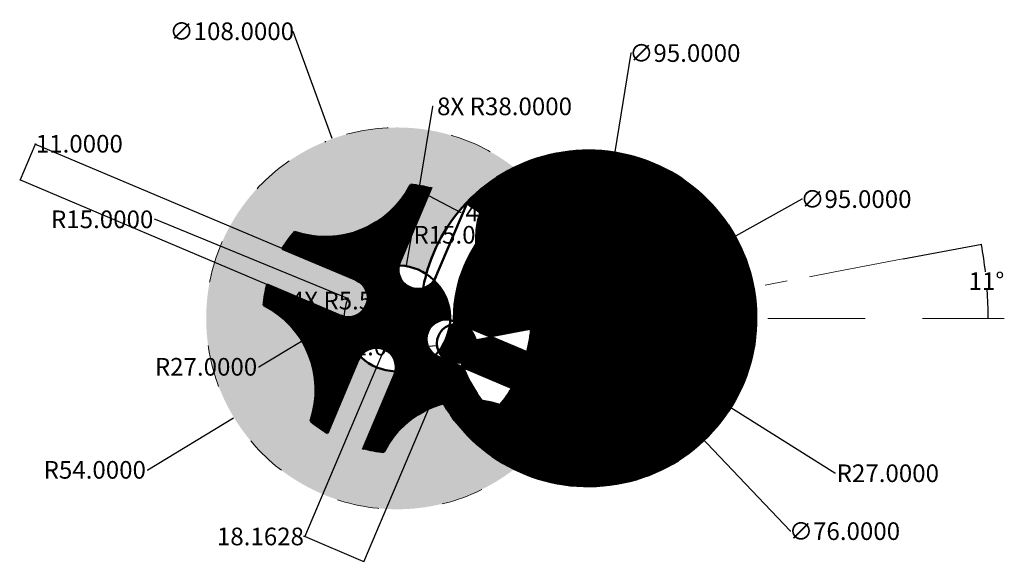
# Model space of a CAD drawing. Units: inches. Extents: x 60331 to 60609, y 22624 to 22778.
import ezdxf

# ---------------------------------------------------------------- set-up
doc = ezdxf.new("R2010")
doc.units = ezdxf.units.IN
doc.header["$MEASUREMENT"] = 0
doc.linetypes.add('ACAD_ISO03W100', pattern=[30, 12, -18])
doc.linetypes.add('CENTER', pattern=[50.8, 31.75, -6.35, 6.35, -6.35])
for name, color, linetype, lineweight in [('M-CNTR', 4, 'CENTER', 18), ('M-CONS', 8, 'ACAD_ISO03W100', 13), ('M-DIMS', 2, 'Continuous', 25), ('M-HATC', 252, 'Continuous', 18), ('M-OUTL', 7, 'Continuous', 50)]:
    doc.layers.add(name, color=color, linetype=linetype, lineweight=lineweight)
doc.styles.get("Standard").update_dxf_attribs({"font": 'arial.ttf'})
doc.dimstyles.get("Standard").update_dxf_attribs({"dimtxt": 5, "dimasz": 0.18, "dimexe": 0.18, "dimexo": 0.0625, "dimgap": 0.09, "dimtad": 0, "dimtih": 1, "dimtoh": 1, "dimdec": 4, "dimzin": 0, "dimdsep": 46, "dimtxsty": 'Standard', "dimcen": 0.09, "dimadec": 0, "dimazin": 0, "dimtfac": 1, "dimtdec": 4, "dimtofl": 0, "dimtmove": 0, "dimatfit": 3, "dimfxl": 1, "dimtolj": 1, "dimtzin": 0, "dimarcsym": 0})

# ---------------------------------------------------------------- blocks, each defined once
blk = doc.blocks.new('*D1')
at = {"layer": 'Defpoints', "color": 0, "transparency": 16777216}
for p in [(60532.97, 22716.4), (60450.04, 22670.06)]:
    blk.add_point(p, dxfattribs=at)
at = {"layer": 'M-DIMS', "color": 0, "lineweight": -2, "transparency": 16777216}
for p, q in [((60551.88, 22726.97), (60533.12, 22716.49)), ((60552.06, 22726.97), (60551.88, 22726.97)), ((60491.41, 22693.23), (60491.59, 22693.23)), ((60491.5, 22693.14), (60491.5, 22693.32))]:
    blk.add_line(p, q, dxfattribs=at)
at = {"layer": 'M-DIMS', "color": 0, "transparency": 16777216}
blk.add_solid([(60533.11, 22716.52), (60533.14, 22716.46), (60532.97, 22716.4)], dxfattribs=at)
at = {"layer": 'M-DIMS', "color": 0, "transparency": 16777216, "insert": (60567.18, 22726.97), "char_height": 5, "attachment_point": 5}
blk.add_mtext('\\A1;∅95.0000', dxfattribs=at)
blk = doc.blocks.new('*D2')
at = {"layer": 'Defpoints', "color": 0, "transparency": 16777216}
for p in [(60580.44, 22710.03), (60561.22, 22706.39), (60604.35, 22700.25), (60586.01, 22693.22), (60609.08, 22693.22)]:
    blk.add_point(p, dxfattribs=at)
at = {"layer": 'M-DIMS', "color": 0, "lineweight": -2, "transparency": 16777216}
blk.add_line((60580.5, 22710.04), (60602.78, 22714.25), dxfattribs=at)
for start, end in [(6.6776, 10.6133), (0.0912, 4.0298)]:
    blk.add_arc((60491.54, 22693.22), 113.04, start, end, dxfattribs=at)
at = {"layer": 'M-DIMS', "color": 0, "transparency": 16777216}
for points in [[(60602.61, 22714.03), (60602.67, 22714.04), (60602.61, 22714.22)], [(60604.6, 22693.4), (60604.54, 22693.4), (60604.57, 22693.22)]]:
    blk.add_solid(points, dxfattribs=at)
at = {"layer": 'M-DIMS', "color": 0, "transparency": 16777216, "insert": (60604.08, 22703.76), "char_height": 5, "attachment_point": 5}
blk.add_mtext('\\A1;11°', dxfattribs=at)
blk = doc.blocks.new('*D3')
at = {"layer": 'Defpoints', "color": 0, "transparency": 16777216}
for p in [(60491.5, 22693.23), (60514.36, 22678.87)]:
    blk.add_point(p, dxfattribs=at)
at = {"layer": 'M-DIMS', "color": 0, "lineweight": -2, "transparency": 16777216}
for p, q in [((60491.41, 22693.23), (60491.59, 22693.23)), ((60491.5, 22693.14), (60491.5, 22693.32)), ((60561.22, 22649.42), (60514.52, 22678.77)), ((60561.4, 22649.42), (60561.22, 22649.42))]:
    blk.add_line(p, q, dxfattribs=at)
at = {"layer": 'M-DIMS', "color": 0, "transparency": 16777216}
blk.add_solid([(60514.53, 22678.8), (60514.5, 22678.74), (60514.36, 22678.87)], dxfattribs=at)
at = {"layer": 'M-DIMS', "color": 0, "transparency": 16777216, "insert": (60576.19, 22649.42), "char_height": 5, "attachment_point": 5}
blk.add_mtext('\\A1;R27.0000', dxfattribs=at)
blk = doc.blocks.new('*D4')
at = {"layer": 'Defpoints', "color": 0, "transparency": 16777216}
for p in [(60465.34, 22720.79), (60517.66, 22665.67)]:
    blk.add_point(p, dxfattribs=at)
at = {"layer": 'M-DIMS', "color": 0, "lineweight": -2, "transparency": 16777216}
for p, q in [((60491.41, 22693.23), (60491.59, 22693.23)), ((60491.5, 22693.14), (60491.5, 22693.32)), ((60548.63, 22633.04), (60517.79, 22665.54)), ((60548.81, 22633.04), (60548.63, 22633.04))]:
    blk.add_line(p, q, dxfattribs=at)
at = {"layer": 'M-DIMS', "color": 0, "transparency": 16777216}
blk.add_solid([(60517.81, 22665.56), (60517.76, 22665.52), (60517.66, 22665.67)], dxfattribs=at)
at = {"layer": 'M-DIMS', "color": 0, "transparency": 16777216, "insert": (60563.94, 22633.04), "char_height": 5, "attachment_point": 5}
blk.add_mtext('\\A1;∅76.0000', dxfattribs=at)
blk = doc.blocks.new('*D5')
at = {"layer": 'Defpoints', "color": 0, "transparency": 16777216}
for p in [(60437.44, 22693.23), (60454.17, 22686.16), (60411.31, 22631.47)]:
    blk.add_point(p, dxfattribs=at)
at = {"layer": 'M-DIMS', "color": 0, "lineweight": -2, "transparency": 16777216}
for p, q in [((60437.41, 22693.17), (60411.24, 22631.3)), ((60454.14, 22686.1), (60427.97, 22624.23)), ((60411.15, 22631.54), (60410.97, 22631.54)), ((60411.31, 22631.47), (60411.15, 22631.54)), ((60427.87, 22624.46), (60411.48, 22631.4))]:
    blk.add_line(p, q, dxfattribs=at)
at = {"layer": 'M-DIMS', "color": 0, "transparency": 16777216}
for points in [[(60411.49, 22631.43), (60411.47, 22631.37), (60411.31, 22631.47)], [(60427.89, 22624.49), (60427.86, 22624.43), (60428.04, 22624.39)]]:
    blk.add_solid(points, dxfattribs=at)
at = {"layer": 'M-DIMS', "color": 0, "transparency": 16777216, "insert": (60398.79, 22631.54), "char_height": 5, "attachment_point": 5}
blk.add_mtext('\\A1;18.1628', dxfattribs=at)
blk = doc.blocks.new('*D6')
at = {"layer": 'Defpoints', "color": 0, "transparency": 16777216}
for p in [(60423.56, 22698.92), (60437.44, 22693.23)]:
    blk.add_point(p, dxfattribs=at)
at = {"layer": 'M-DIMS', "color": 0, "lineweight": -2, "transparency": 16777216}
for p, q in [((60368.83, 22721.25), (60369.01, 22721.25)), ((60369.01, 22721.25), (60423.39, 22698.98)), ((60437.35, 22693.23), (60437.53, 22693.23)), ((60437.44, 22693.14), (60437.44, 22693.32))]:
    blk.add_line(p, q, dxfattribs=at)
blk.add_arc((60437.44, 22693.23), 15, 157.0434, 177.9603, dxfattribs=at)
at = {"layer": 'M-DIMS', "color": 0, "transparency": 16777216}
blk.add_solid([(60423.4, 22699.01), (60423.38, 22698.96), (60423.56, 22698.92)], dxfattribs=at)
at = {"layer": 'M-DIMS', "color": 0, "transparency": 16777216, "insert": (60354.03, 22721.25), "char_height": 5, "attachment_point": 5}
blk.add_mtext('\\A1;R15.0000', dxfattribs=at)
blk = doc.blocks.new('*D7')
at = {"layer": 'Defpoints', "color": 0, "transparency": 16777216}
for p in [(60410.55, 22686.83), (60387.4, 22672.94)]:
    blk.add_point(p, dxfattribs=at)
at = {"layer": 'M-DIMS', "color": 0, "lineweight": -2, "transparency": 16777216}
for p, q in [((60398.37, 22679.53), (60410.39, 22686.74)), ((60398.19, 22679.53), (60398.37, 22679.53))]:
    blk.add_line(p, q, dxfattribs=at)
at = {"layer": 'M-DIMS', "color": 0, "transparency": 16777216}
blk.add_solid([(60410.38, 22686.76), (60410.41, 22686.71), (60410.55, 22686.83)], dxfattribs=at)
at = {"layer": 'M-DIMS', "color": 0, "transparency": 16777216, "insert": (60383.4, 22679.53), "char_height": 5, "attachment_point": 5}
blk.add_mtext('\\A1;R27.0000', dxfattribs=at)
blk = doc.blocks.new('*D8')
at = {"layer": 'Defpoints', "color": 0, "transparency": 16777216}
for p in [(60437.44, 22693.23), (60391.29, 22665.19)]:
    blk.add_point(p, dxfattribs=at)
at = {"layer": 'M-DIMS', "color": 0, "lineweight": -2, "transparency": 16777216}
for p, q in [((60437.35, 22693.23), (60437.53, 22693.23)), ((60437.44, 22693.14), (60437.44, 22693.32)), ((60366.91, 22650.38), (60391.14, 22665.1)), ((60366.73, 22650.38), (60366.91, 22650.38))]:
    blk.add_line(p, q, dxfattribs=at)
at = {"layer": 'M-DIMS', "color": 0, "transparency": 16777216}
blk.add_solid([(60391.12, 22665.12), (60391.15, 22665.07), (60391.29, 22665.19)], dxfattribs=at)
at = {"layer": 'M-DIMS', "color": 0, "transparency": 16777216, "insert": (60351.94, 22650.38), "char_height": 5, "attachment_point": 5}
blk.add_mtext('\\A1;R54.0000', dxfattribs=at)
blk = doc.blocks.new('*D9')
at = {"layer": 'Defpoints', "color": 0, "transparency": 16777216}
for p in [(60335.16, 22742.47), (60404.95, 22712.95), (60400.67, 22702.81)]:
    blk.add_point(p, dxfattribs=at)
at = {"layer": 'M-DIMS', "color": 0, "lineweight": -2, "transparency": 16777216}
for p, q in [((60330.95, 22732.5), (60335.09, 22742.3)), ((60404.9, 22712.97), (60335, 22742.54)), ((60335.16, 22742.47), (60335.23, 22742.63)), ((60335.23, 22742.63), (60335.41, 22742.63)), ((60400.61, 22702.84), (60330.71, 22732.41))]:
    blk.add_line(p, q, dxfattribs=at)
at = {"layer": 'M-DIMS', "color": 0, "transparency": 16777216}
for points in [[(60335.06, 22742.31), (60335.12, 22742.29), (60335.16, 22742.47)], [(60330.92, 22732.51), (60330.97, 22732.49), (60330.88, 22732.34)]]:
    blk.add_solid(points, dxfattribs=at)
at = {"layer": 'M-DIMS', "color": 0, "transparency": 16777216, "insert": (60347.58, 22742.63), "char_height": 5, "attachment_point": 5}
blk.add_mtext('\\A1;11.0000', dxfattribs=at)
blk = doc.blocks.new('*D10')
at = {"layer": 'Defpoints', "color": 0, "transparency": 16777216}
for p in [(60419, 22743.99), (60455.88, 22642.48)]:
    blk.add_point(p, dxfattribs=at)
at = {"layer": 'M-DIMS', "color": 0, "lineweight": -2, "transparency": 16777216}
for p, q in [((60407.76, 22774.44), (60407.94, 22774.44)), ((60407.94, 22774.44), (60418.94, 22744.16)), ((60437.35, 22693.23), (60437.53, 22693.23)), ((60437.44, 22693.14), (60437.44, 22693.32))]:
    blk.add_line(p, q, dxfattribs=at)
at = {"layer": 'M-DIMS', "color": 0, "transparency": 16777216}
blk.add_solid([(60418.97, 22744.17), (60418.91, 22744.15), (60419, 22743.99)], dxfattribs=at)
at = {"layer": 'M-DIMS', "color": 0, "transparency": 16777216, "insert": (60390.69, 22774.44), "char_height": 5, "attachment_point": 5}
blk.add_mtext('\\A1;∅108.0000', dxfattribs=at)
blk = doc.blocks.new('*D11')
at = {"layer": 'Defpoints', "color": 0, "transparency": 16777216}
for p in [(60499, 22740.14), (60484, 22646.33)]:
    blk.add_point(p, dxfattribs=at)
at = {"layer": 'M-DIMS', "color": 0, "lineweight": -2, "transparency": 16777216}
for p, q in [((60503.5, 22768.28), (60499.03, 22740.31)), ((60503.68, 22768.28), (60503.5, 22768.28)), ((60491.41, 22693.23), (60491.59, 22693.23)), ((60491.5, 22693.14), (60491.5, 22693.32))]:
    blk.add_line(p, q, dxfattribs=at)
at = {"layer": 'M-DIMS', "color": 0, "transparency": 16777216}
blk.add_solid([(60499, 22740.32), (60499.06, 22740.31), (60499, 22740.14)], dxfattribs=at)
at = {"layer": 'M-DIMS', "color": 0, "transparency": 16777216, "insert": (60518.8, 22768.28), "char_height": 5, "attachment_point": 5}
blk.add_mtext('\\A1;∅95.0000', dxfattribs=at)
blk = doc.blocks.new('*D12')
at = {"layer": 'Defpoints', "color": 0, "transparency": 16777216}
for p in [(60417.15, 22743.27), (60441.04, 22730.7)]:
    blk.add_point(p, dxfattribs=at)
at = {"layer": 'M-DIMS', "color": 0, "lineweight": -2, "transparency": 16777216}
for p, q in [((60417.06, 22743.27), (60417.24, 22743.27)), ((60417.15, 22743.18), (60417.15, 22743.36)), ((60455.38, 22723.16), (60441.2, 22730.62)), ((60455.56, 22723.16), (60455.38, 22723.16))]:
    blk.add_line(p, q, dxfattribs=at)
at = {"layer": 'M-DIMS', "color": 0, "transparency": 16777216}
blk.add_solid([(60441.22, 22730.64), (60441.19, 22730.59), (60441.04, 22730.7)], dxfattribs=at)
at = {"layer": 'M-DIMS', "color": 0, "transparency": 16777216, "insert": (60475.83, 22723.16), "char_height": 5, "attachment_point": 5}
blk.add_mtext('\\A1;4X R27.0000', dxfattribs=at)
blk = doc.blocks.new('*D13')
at = {"layer": 'Defpoints', "color": 0, "transparency": 16777216}
for p in [(60440, 22708.01), (60437.44, 22693.23)]:
    blk.add_point(p, dxfattribs=at)
at = {"layer": 'M-DIMS', "color": 0, "lineweight": -2, "transparency": 16777216}
for p, q in [((60441.54, 22716.88), (60440.03, 22708.19)), ((60441.72, 22716.88), (60441.54, 22716.88)), ((60437.35, 22693.23), (60437.53, 22693.23)), ((60437.44, 22693.14), (60437.44, 22693.32))]:
    blk.add_line(p, q, dxfattribs=at)
at = {"layer": 'M-DIMS', "color": 0, "transparency": 16777216}
blk.add_solid([(60440, 22708.19), (60440.06, 22708.18), (60440, 22708.01)], dxfattribs=at)
at = {"layer": 'M-DIMS', "color": 0, "transparency": 16777216, "insert": (60456.51, 22716.88), "char_height": 5, "attachment_point": 5}
blk.add_mtext('\\A1;R15.0000', dxfattribs=at)
blk = doc.blocks.new('*D14')
at = {"layer": 'Defpoints', "color": 0, "transparency": 16777216}
for p in [(60443.28, 22707.05), (60443.15, 22701.55)]:
    blk.add_point(p, dxfattribs=at)
at = {"layer": 'M-DIMS', "color": 0, "lineweight": -2, "transparency": 16777216}
for p, q in [((60443.19, 22707.05), (60443.37, 22707.05)), ((60443.28, 22706.96), (60443.28, 22707.14)), ((60443.07, 22698.25), (60443.14, 22701.37)), ((60442.89, 22698.25), (60443.07, 22698.25))]:
    blk.add_line(p, q, dxfattribs=at)
at = {"layer": 'M-DIMS', "color": 0, "transparency": 16777216}
blk.add_solid([(60443.11, 22701.37), (60443.17, 22701.37), (60443.15, 22701.55)], dxfattribs=at)
at = {"layer": 'M-DIMS', "color": 0, "transparency": 16777216, "insert": (60424.56, 22698.25), "char_height": 5, "attachment_point": 5}
blk.add_mtext('\\A1;4X R5.5000', dxfattribs=at)
blk = doc.blocks.new('*D15')
at = {"layer": 'Defpoints', "color": 0, "transparency": 16777216}
for p in [(60448.69, 22685.6), (60459.64, 22686.71)]:
    blk.add_point(p, dxfattribs=at)
at = {"layer": 'M-DIMS', "color": 0, "lineweight": -2, "transparency": 16777216}
for p, q in [((60445.41, 22685.27), (60448.52, 22685.58)), ((60454.08, 22686.16), (60454.26, 22686.16)), ((60454.17, 22686.07), (60454.17, 22686.25))]:
    blk.add_line(p, q, dxfattribs=at)
at = {"layer": 'M-DIMS', "color": 0, "transparency": 16777216}
blk.add_solid([(60448.51, 22685.61), (60448.52, 22685.55), (60448.69, 22685.6)], dxfattribs=at)
at = {"layer": 'M-DIMS', "color": 0, "transparency": 16777216, "insert": (60430.29, 22685.27), "char_height": 5, "attachment_point": 5}
blk.add_mtext('\\A1;∅11.0000', dxfattribs=at)
blk = doc.blocks.new('*D16')
at = {"layer": 'Defpoints', "color": 0, "transparency": 16777216}
for p in [(60443.7, 22730.71), (60437.44, 22693.23)]:
    blk.add_point(p, dxfattribs=at)
at = {"layer": 'M-DIMS', "color": 0, "lineweight": -2, "transparency": 16777216}
for p, q in [((60447.46, 22753.2), (60443.73, 22730.89)), ((60447.64, 22753.2), (60447.46, 22753.2)), ((60437.35, 22693.23), (60437.53, 22693.23)), ((60437.44, 22693.14), (60437.44, 22693.32))]:
    blk.add_line(p, q, dxfattribs=at)
at = {"layer": 'M-DIMS', "color": 0, "transparency": 16777216}
blk.add_solid([(60443.7, 22730.89), (60443.76, 22730.88), (60443.7, 22730.71)], dxfattribs=at)
at = {"layer": 'M-DIMS', "color": 0, "transparency": 16777216, "insert": (60467.81, 22753.2), "char_height": 5, "attachment_point": 5}
blk.add_mtext('\\A1;8X R38.0000', dxfattribs=at)

msp = doc.modelspace()

# ---------------------------------------------------------------- hatches: boundary and pattern name
at = {"layer": 'M-HATC'}
h = msp.add_hatch(color=256, dxfattribs=at)
h.dxf.hatch_style = 1
h.paths.add_polyline_path([(60383.4389, 22693.23138, 0.62395168), (60470.57212, 22650.59115, -0.147115616), (60450.52409, 22669.20932, 0.210663072), (60433.65907, 22655.41984, -0.038845732), (60427.85582, 22656.45959), (60436.66049, 22677.27381, 0.04612672), (60436.96747, 22678.23879, -0.186494261), (60427.00831, 22682.45164, 0.04612672), (60426.52962, 22681.5593), (60417.72495, 22660.74508, -0.038845732), (60412.93719, 22664.18545, 0.373805178), (60399.62735, 22697.01121, -0.038845732), (60400.66711, 22702.81446), (60421.48133, 22694.00979, 0.04612672), (60422.44631, 22693.70281, 0.911814278), (60425.76681, 22704.14066), (60404.95259, 22712.94533, -0.038845732), (60408.39296, 22717.73309, 0.373805178), (60441.21873, 22731.04293, -0.038845732), (60447.02197, 22730.00318), (60438.2173, 22709.18896, 0.04612672), (60437.91032, 22708.22398, -0.138521755), (60445.68454, 22705.76172, -0.12300399), (60456.9584, 22725.8349, -0.089735654), (60470.57212, 22735.87162, 0.62395168)])
h.paths.add_polyline_path([(60366.8953, 22674.3393), (60399.68861, 22674.3393), (60399.68861, 22684.64284), (60366.8953, 22684.64284)], flags=9)
h = msp.add_hatch(dxfattribs=at)
h.set_pattern_fill('ANSI31', color=256)
h.paths.add_polyline_path([(60484.69682, 22719.35971, -0.126939701), (60491.4389, 22693.23138), (60491.59938, 22693.23138), (60518.03552, 22698.2287, 0.434461621)])
h.paths.add_polyline_path([(60484.69682, 22719.35971, 0.18019045), (60469.26217, 22708.54117, -0.200284197), (60480.6968, 22691.17043), (60491.43889, 22693.20105, 0.127082418)])
h.paths.add_polyline_path([(60518.50201, 22693.21942), (60491.5361, 22693.21942), (60491.43889, 22693.20105, -0.126796988), (60484.69682, 22667.10306, 0.490832057)], flags=17)
h.paths.add_polyline_path([(60491.43889, 22693.20105), (60480.6968, 22691.17043, -0.200036708), (60476.40649, 22670.84556, 0.084827533), (60484.69682, 22667.10306, 0.126796988)], flags=17)
h.paths.add_polyline_path([(60518.03552, 22698.2287), (60491.5361, 22693.21942), (60518.50201, 22693.21942, 0.046684438)])
h.paths.add_polyline_path([(60470.57212, 22735.87162, -0.047925325), (60478.08417, 22728.78362, -0.466306924), (60528.8441, 22700.27189), (60538.17878, 22702.03646, 0.495650446)])
h.paths.add_polyline_path([(60539.00201, 22693.21942), (60529.50201, 22693.21942, -0.524227578), (60478.08417, 22657.67915, -0.047925325), (60470.57212, 22650.59115, 0.555048595)])
h.paths.add_polyline_path([(60461.4879, 22669.92575, 0.102808528), (60450.52409, 22669.20932, 0.147115616), (60470.57212, 22650.59115, 0.047925325), (60478.08417, 22657.67915, -0.138289792)])
h.paths.add_polyline_path([(60478.08417, 22728.78362, 0.047925325), (60470.57212, 22735.87162, 0.089735654), (60456.9584, 22725.8349, -0.031670848), (60460.92, 22723.10843, 0.084312993), (60459.77152, 22714.14014, -0.158116424)])
h.paths.add_polyline_path([(60538.17878, 22702.03646), (60528.8441, 22700.27189, -0.046700883), (60529.50201, 22693.21942), (60539.00201, 22693.21942, 0.046708956)])
h = msp.add_hatch(dxfattribs=at)
h.set_pattern_fill('ANSI31', color=256)
h.paths.add_polyline_path([(60447.02197, 22730.00318, 0.038845732), (60441.21873, 22731.04293, -0.373805178), (60408.39296, 22717.73309, 0.038845732), (60404.95259, 22712.94533), (60426.72898, 22703.73365, -0.207907545), (60437.81029, 22708.22679)])
h.paths.add_polyline_path([(60422.4435, 22693.60278), (60400.66711, 22702.81446, 0.038845732), (60399.62735, 22697.01121, -0.373805178), (60412.93719, 22664.18545, 0.038845732), (60417.72495, 22660.74508), (60426.93663, 22682.52147, -0.207907545)])
h.paths.add_polyline_path([(60456.12643, 22679.35449), (60448.14882, 22682.72912, -0.207907545), (60437.0675, 22678.23598), (60427.85582, 22656.45959, 0.038845732), (60433.65907, 22655.41984, -0.32041105), (60461.4879, 22669.92575, -0.071725624)])
h.paths.add_polyline_path([(60459.77152, 22714.14014, 0.14669898), (60453.50201, 22693.23138, 0.00544033), (60453.51101, 22692.40453), (60456.30939, 22691.22078), (60463.92383, 22687.99978), (60475.31399, 22690.1529, 0.004026541), (60475.35866, 22690.76329, -0.280647131)])
h = msp.add_hatch(dxfattribs=at)
h.set_pattern_fill('ANSI31', color=256)
h.paths.add_polyline_path([(60478.08417, 22728.78362, -0.053450789), (60484.69682, 22719.35971, -0.434461621), (60518.03552, 22698.2287), (60528.8441, 22700.27189, 0.466306924)])
h.paths.add_polyline_path([(60528.8441, 22700.27189), (60518.03552, 22698.2287, -0.046684438), (60518.50201, 22693.21942), (60529.50201, 22693.21942, 0.046700883)])
h.paths.add_polyline_path([(60529.50201, 22693.21942), (60518.50201, 22693.21942, -0.490832057), (60484.69682, 22667.10306, -0.053450789), (60478.08417, 22657.67915, 0.524227578)])
h.paths.add_polyline_path([(60484.69682, 22667.10306, -0.084827533), (60476.40649, 22670.84556, 0.200036708), (60480.6968, 22691.17043), (60475.31399, 22690.1529, -0.043486667), (60474.21069, 22683.64831), (60463.92383, 22687.99978), (60459.57094, 22687.17693, -0.046741248), (60459.66665, 22686.15534, -0.340029462), (60455.57919, 22680.83983, 0.010415234), (60456.12643, 22679.35449), (60469.92521, 22673.51744, -0.038845732), (60466.48484, 22668.72968, 0.047683064), (60461.4879, 22669.92575, 0.138289792), (60478.08417, 22657.67915, 0.053450789)])
h.paths.add_polyline_path([(60469.26217, 22708.54117, -0.18019045), (60484.69682, 22719.35971, 0.053450789), (60478.08417, 22728.78362, 0.158116424), (60459.77152, 22714.14014, 0.280647131), (60475.35866, 22690.76329, -0.004026541), (60475.31399, 22690.1529), (60480.6968, 22691.17043, 0.200284197)])
h = msp.add_hatch(dxfattribs=at)
h.set_pattern_fill('ANSI31', color=256)
h.paths.add_polyline_path([(60437.91032, 22708.22398, 0.211389769), (60426.65916, 22703.66197, -0.830747161), (60422.44631, 22693.70281, 0.211389769), (60427.00831, 22682.45164, -0.830747161), (60436.96747, 22678.23879, 0.211389769), (60448.21864, 22682.8008, -0.830747161), (60452.43149, 22692.75996, 0.211389769), (60447.86949, 22704.01113, -0.830747161)])
h = msp.add_hatch(dxfattribs=at)
h.set_pattern_fill('ANSI31', color=256)
h.paths.add_polyline_path([(60453.53623, 22691.61909, 0.036231711), (60454.16665, 22686.15534), (60459.57094, 22687.17693, 0.393291825)])
h.paths.add_polyline_path([(60453.53623, 22691.61909, 0.057011752), (60452.31861, 22691.33557, -0.137588095), (60449.16219, 22683.8738, 0.36581681), (60455.57919, 22680.83983, -0.072558672)])
h.paths.add_polyline_path([(60459.66665, 22686.15534, 0.046741248), (60459.57094, 22687.17693), (60454.16665, 22686.15534, 0.036231711), (60455.57919, 22680.83983, 0.340029462)])

# ---------------------------------------------------------------- linework, layer by layer
at = {"layer": 'M-CNTR'}
for p, q in [((60561.21921, 22706.39187), (60580.43989, 22710.02522)), ((60454.16665, 22686.15534), (60561.21921, 22706.39187)), ((60491.4389, 22693.21942), (60569.80006, 22693.21942)), ((60586.00818, 22693.21942), (60609.08109, 22693.21942))]:
    msp.add_line(p, q, dxfattribs=at)
at = {"layer": 'M-CONS'}
for p, q in [((60491.50201, 22693.23138), (60491.4389, 22693.23138)), ((60491.4389, 22693.21942), (60491.50201, 22693.23138))]:
    msp.add_line(p, q, dxfattribs=at)
msp.add_circle((60437.4389, 22693.23138), 54, dxfattribs=at)
at = {"layer": 'M-OUTL'}
for p, q in [((60447.17786, 22730.37169), (60437.81029, 22708.22679)), ((60457.30873, 22726.08621), (60447.94117, 22703.9413)), ((60426.72898, 22703.73365), (60404.95259, 22712.94533)), ((60422.4435, 22693.60278), (60400.66711, 22702.81446)), ((60456.30939, 22691.22078), (60453.39647, 22692.45298)), ((60474.21069, 22683.64831), (60456.30939, 22691.22078)), ((60469.92521, 22673.51744), (60448.14882, 22682.72912)), ((60426.93663, 22682.52147), (60417.72495, 22660.74508)), ((60437.0675, 22678.23598), (60427.69994, 22656.09107))]:
    msp.add_line(p, q, dxfattribs=at)
for centre, radius in [((60491.50201, 22693.23138), 38), ((60454.16665, 22686.15534), 5.5)]:
    msp.add_circle(centre, radius, dxfattribs=at)
for centre, radius, start, end in [((60491.50201, 22693.23138), 47.5, 210.3796727, 136.6550024), ((60417.14808, 22743.27419), 27, 251.0790377, 333.0630515), ((60437.4389, 22693.23138), 38, 75.3930852, 84.2913971), ((60491.50201, 22693.23138), 47.5, 136.6550024, 169.6665105), ((60437.4389, 22693.23138), 38, 51.835325, 59.0913234), ((60486.74899, 22715.24309), 27, 163.0636706, 245.0476844), ((60491.50201, 22693.23138), 27, 236.0068686, 145.4566949), ((60437.4389, 22693.23138), 38, 139.8506921, 148.749004), ((60437.4389, 22693.23138), 15, 178.1989998, 135.9430894), ((60443.28274, 22707.04621), 5.5, 157.0710446, 326.507067), ((60443.28274, 22707.04621), 5.5, 157.0710446, 167.6350222), ((60454.16665, 22686.15534), 27, 325.4566949, 56.0068686), ((60437.4389, 22693.23138), 38, 165.3930852, 174.2913971), ((60423.62407, 22699.07523), 5.5, 247.0710446, 67.0710446), ((60423.62407, 22699.07523), 5.5, 56.507067, 67.0710446), ((60443.28274, 22707.04621), 5.5, 326.507067, 337.0710446), ((60387.39609, 22672.94056), 27, 341.0790377, 63.0630515), ((60423.62407, 22699.07523), 5.5, 247.0710446, 257.6350222), ((60451.25373, 22687.38754), 5.5, 67.0710446, 247.0710446), ((60437.4389, 22693.23138), 38, 345.3930852, 356.27603), ((60431.59506, 22679.41656), 5.5, 337.0710446, 157.0710446), ((60431.59506, 22679.41656), 5.5, 146.507067, 157.0710446), ((60431.59506, 22679.41656), 5.5, 337.0710446, 347.6350222), ((60437.4389, 22693.23138), 38, 319.8506921, 328.749004), ((60457.72972, 22643.18858), 27, 71.0790377, 153.0630515), ((60437.4389, 22693.23138), 38, 229.8506921, 238.749004), ((60437.4389, 22693.23138), 38, 255.3930852, 264.2913971)]:
    msp.add_arc(centre, radius, start, end, dxfattribs=at)

# ---------------------------------------------------------------- dimensions: what is measured, and where the dimension line sits
at = {"layer": 'M-DIMS'}
for p1, p2, override, picture, middle in [((60455.87644, 22642.47651), (60419.00136, 22743.98626), {"dimdec": 4, "dimlfac": 1, "dimrnd": 0, "dimzin": 0, "dimdsep": 46, "dimlunit": 2}, '*D10', (60390.69407, 22774.43918)), ((60484.00312, 22646.32705), (60499.00091, 22740.13572), {"dimdec": 4, "dimlfac": 1, "dimrnd": 0, "dimzin": 0, "dimdsep": 46, "dimlunit": 2}, '*D11', (60518.80265, 22768.27832)), ((60450.03714, 22670.05998), (60532.96689, 22716.40279), {"dimclrd": 0, "dimclre": 0, "dimclrt": 0}, '*D1', (60567.17799, 22726.96935)), ((60465.34221, 22720.7934), (60517.66182, 22665.66937), {"dimclrd": 0, "dimclre": 0, "dimclrt": 0}, '*D4', (60563.9364, 22633.03704)), ((60459.63849, 22686.71121), (60448.69481, 22685.59947), {"dimdec": 4, "dimlfac": 1, "dimrnd": 0, "dimzin": 0, "dimdsep": 46, "dimlunit": 2}, '*D15', (60445.41171, 22685.26595))]:
    dim = msp.add_diameter_dim_2p(p1=p1, p2=p2, dimstyle='Standard', override=override, dxfattribs=at)
    dim.commit()
    dim.dimension.update_dxf_attribs({"geometry": picture, "text_midpoint": middle, "dimtype": 163})
for center, mpoint, text, picture, middle in [((60437.4389, 22693.23138), (60443.70033, 22730.71197), '8X <>', '*D16', (60467.80734, 22753.20033)), ((60417.14807, 22743.27419), (60441.04216, 22730.7015), '4X <>', '*D12', (60475.82597, 22723.15789)), ((60443.28274, 22707.04621), (60443.14749, 22701.54788), '4X <>', '*D14', (60424.56134, 22698.24888))]:
    dim = msp.add_radius_dim(center=center, mpoint=mpoint, text=text, dimstyle='Standard', override={"dimdec": 4, "dimlfac": 1, "dimrnd": 0, "dimzin": 0, "dimdsep": 46, "dimlunit": 2}, dxfattribs=at)
    dim.commit()
    dim.dimension.update_dxf_attribs({"geometry": picture, "text_midpoint": middle, "dimtype": 164})
for p1, p2, distance, picture, middle in [((60400.66711, 22702.81446), (60404.95259, 22712.94533), 75.77908, '*D9', (60347.57812, 22742.63384)), ((60454.16665, 22686.15534), (60437.4389, 22693.23138), 67.06219, '*D5', (60398.78567, 22631.53799))]:
    dim = msp.add_aligned_dim(p1=p1, p2=p2, distance=distance, dimstyle='Standard', override={"dimclrd": 0, "dimclre": 0, "dimclrt": 0}, dxfattribs=at)
    dim.commit()
    dim.dimension.update_dxf_attribs({"geometry": picture, "text_midpoint": middle})
for center, mpoint, override, picture, middle in [((60437.4389, 22693.23138), (60423.55768, 22698.91572), {"dimclrd": 0, "dimclre": 0, "dimclrt": 0}, '*D6', (60354.03395, 22721.25334)), ((60437.4389, 22693.23138), (60440.00019, 22708.01109), {"dimdec": 4, "dimlfac": 1, "dimrnd": 0, "dimzin": 0, "dimdsep": 46, "dimlunit": 2}, '*D13', (60456.51194, 22716.87892)), ((60437.4389, 22693.23138), (60391.29073, 22665.18951), {"dimclrd": 0, "dimclre": 0, "dimclrt": 0}, '*D8', (60351.93644, 22650.37545)), ((60491.50201, 22693.23138), (60514.36322, 22678.86597), {"dimclrd": 0, "dimclre": 0, "dimclrt": 0}, '*D3', (60576.19419, 22649.42282)), ((60387.39609, 22672.94056), (60410.549, 22686.83094), {"dimclrd": 0, "dimclre": 0, "dimclrt": 0}, '*D7', (60383.39939, 22679.52688))]:
    dim = msp.add_radius_dim(center=center, mpoint=mpoint, dimstyle='Standard', override=override, dxfattribs=at)
    dim.commit()
    dim.dimension.update_dxf_attribs({"geometry": picture, "text_midpoint": middle, "dimtype": 164})
dim = msp.add_angular_dim_2l(base=(60604.35378, 22700.25439), line1=((60586.00818, 22693.21942), (60609.08109, 22693.21942)), line2=((60561.21921, 22706.39187), (60580.43989, 22710.02522)), dimstyle='Standard', override={"dimclrd": 0, "dimclre": 0, "dimclrt": 0}, dxfattribs=at)
dim.commit()
dim.dimension.update_dxf_attribs({"geometry": '*D2', "text_midpoint": (60604.08007, 22703.76335)})

doc.saveas('drawing.dxf')
